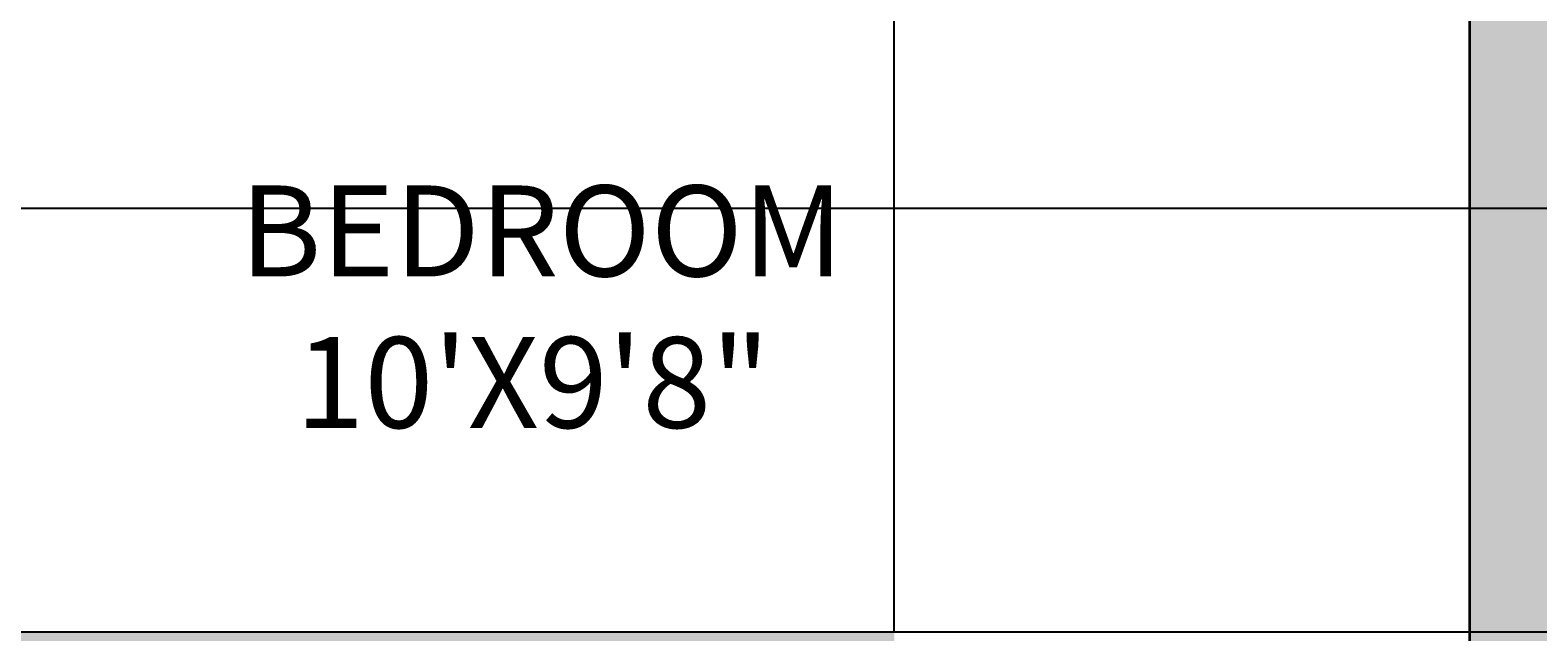
# Model space of a CAD drawing. Units: inches. Extents: x 311 to 815, y -527 to 136.
# Tile 18 of 21: x 444 to 544, y -103 to -63. Entities that reach past the tile are written whole.
import ezdxf

# ---------------------------------------------------------------- set-up
doc = ezdxf.new("R2010")
doc.units = ezdxf.units.IN
doc.header["$MEASUREMENT"] = 0
for name, color, linetype, lineweight in [('A-ANNO-DIMS', 1, 'Continuous', 18), ('A-AREA-IDEN', 8, 'Continuous', 18), ('A-WALL-PATT', 242, 'Continuous', 13), ('wall', 1, 'Continuous', 35)]:
    doc.layers.add(name, color=color, linetype=linetype, lineweight=lineweight)
doc.styles.get("Standard").update_dxf_attribs({"font": 'arial.ttf'})
doc.dimstyles.get("Standard").update_dxf_attribs({"dimtxt": 0.18, "dimasz": 0.18, "dimexe": 0.18, "dimexo": 0.0625, "dimgap": 0.09, "dimtad": 0, "dimtih": 1, "dimtoh": 1, "dimdec": 1, "dimzin": 0, "dimdsep": 46, "dimlunit": 4, "dimtxsty": 'Standard', "dimcen": 0.09, "dimadec": 0, "dimazin": 0, "dimtfac": 1, "dimtdec": 1, "dimtofl": 0, "dimtmove": 0, "dimatfit": 3, "dimfxl": 1, "dimtolj": 1, "dimtzin": 0, "dimarcsym": 0})

# ---------------------------------------------------------------- blocks, each defined once
blk = doc.blocks.new('*D40')
at = {"layer": 'A-ANNO-DIMS', "color": 0, "lineweight": -2, "transparency": 16777216}
for p, q in [((419.385, -75.128), (754.853, -75.128)), ((754.673, -75.308), (754.673, -88.947)), ((754.673, -102.948), (754.673, -89.308)), ((419.385, -103.128), (754.853, -103.128))]:
    blk.add_line(p, q, dxfattribs=at)
at = {"layer": 'A-ANNO-DIMS', "color": 0, "transparency": 16777216}
for points in [[(754.643, -75.308), (754.703, -75.308), (754.673, -75.128)], [(754.643, -102.948), (754.703, -102.948), (754.673, -103.128)]]:
    blk.add_solid(points, dxfattribs=at)
at = {"layer": 'Defpoints', "color": 0, "transparency": 16777216}
for p in [(419.323, -75.128), (419.323, -103.128), (754.673, -103.128)]:
    blk.add_point(p, dxfattribs=at)
at = {"layer": 'A-ANNO-DIMS', "color": 0, "transparency": 16777216, "insert": (754.673, -89.128), "char_height": 0.18, "attachment_point": 5}
blk.add_mtext('\\A1;2\'-4"', dxfattribs=at)
blk = doc.blocks.new('*D51')
at = {"layer": 'A-ANNO-DIMS', "color": 0, "lineweight": -2, "transparency": 16777216}
for p, q in [((501.323, -103.065), (501.323, 54.402)), ((501.503, 54.222), (519.994, 54.222)), ((539.143, 54.222), (520.652, 54.222)), ((539.323, -112.065), (539.323, 54.402))]:
    blk.add_line(p, q, dxfattribs=at)
at = {"layer": 'A-ANNO-DIMS', "color": 0, "transparency": 16777216}
for points in [[(501.503, 54.252), (501.503, 54.192), (501.323, 54.222)], [(539.143, 54.252), (539.143, 54.192), (539.323, 54.222)]]:
    blk.add_solid(points, dxfattribs=at)
at = {"layer": 'Defpoints', "color": 0, "transparency": 16777216}
for p in [(501.323, 54.222), (501.323, -103.128), (539.323, -112.128)]:
    blk.add_point(p, dxfattribs=at)
at = {"layer": 'A-ANNO-DIMS', "color": 0, "transparency": 16777216, "insert": (520.323, 54.222), "char_height": 0.18, "attachment_point": 5}
blk.add_mtext('\\A1;3\'-2"', dxfattribs=at)

msp = doc.modelspace()

# ---------------------------------------------------------------- hatches: boundary and pattern name
at = {"layer": 'A-WALL-PATT'}
h = msp.add_hatch(color=256, dxfattribs=at)
h.dxf.hatch_style = 1
h.paths.add_polyline_path([(557.823, 21.872), (509.323, 21.872), (509.323, 12.872), (539.323, 12.872), (539.323, -112.128), (548.323, -112.128), (548.323, -58.628), (557.823, -58.628), (557.823, -49.628), (548.323, -49.628), (548.323, 12.872), (557.823, 12.872)])
h.paths.add_polyline_path([(449.323, 21.872), (410.323, 21.872), (410.323, -15.128), (419.323, -15.128), (419.323, 12.872), (449.323, 12.872)])
h.paths.add_polyline_path([(626.823, 21.872), (581.823, 21.872), (581.823, 12.872), (591.323, 12.872), (591.323, -49.628), (581.823, -49.628), (581.823, -58.628), (591.323, -58.628), (591.323, -112.128), (600.323, -112.128), (600.323, 12.872), (626.823, 12.872)])
h.paths.add_polyline_path([(722.323, 21.872), (686.823, 21.872), (686.823, 12.872), (713.323, 12.872), (713.323, -18.128), (722.323, -18.128)])
h.paths.add_polyline_path([(722.323, -42.128), (713.323, -42.128), (713.323, -73.128), (722.323, -73.128)])
h.paths.add_polyline_path([(501.323, -103.128), (419.323, -103.128), (419.323, -75.128), (410.323, -75.128), (410.323, -126.628), (419.323, -126.628), (419.323, -112.128), (492.323, -112.128), (492.323, -143.128), (501.323, -143.128)])
h.paths.add_polyline_path([(548.323, -165.128), (419.323, -165.128), (419.323, -150.628), (410.323, -150.628), (410.323, -202.128), (419.323, -202.128), (419.323, -174.128), (548.323, -174.128)])
h.paths.add_polyline_path([(722.323, -103.128), (636.323, -103.128), (636.323, -112.128), (713.323, -112.128), (713.323, -140.128), (722.323, -140.128)])
h.paths.add_polyline_path([(548.323, -210.128), (539.323, -210.128), (539.323, -290.128), (419.323, -290.128), (419.323, -262.128), (410.323, -262.128), (410.323, -311.568), (419.323, -311.568), (419.323, -299.128), (469.323, -299.128), (469.323, -348.128), (443.323, -348.128), (443.323, -357.128), (478.323, -357.128), (478.323, -299.128), (548.323, -299.128)])
h.paths.add_polyline_path([(722.323, -200.128), (713.323, -200.128), (713.323, -228.128), (609.323, -228.128), (609.323, -237.128), (713.323, -237.128), (713.323, -262.628), (722.323, -262.628)])
h.paths.add_polyline_path([(722.323, -322.628), (713.323, -322.628), (713.323, -348.128), (633.323, -348.128), (633.323, -357.128), (713.323, -357.128), (713.323, -385.128), (722.323, -385.128)])
h.paths.add_polyline_path([(419.323, -335.568), (410.323, -335.568), (410.323, -390.84), (419.323, -390.84)])
h.paths.add_polyline_path([(419.323, -450.84), (410.323, -450.84), (410.323, -482.128), (449.323, -482.128), (449.323, -473.128), (419.323, -473.128)])
h.paths.add_polyline_path([(582.823, -473.128), (548.323, -473.128), (548.323, -348.128), (539.323, -348.128), (539.323, -473.128), (509.323, -473.128), (509.323, -482.128), (582.823, -482.128)])
h.paths.add_polyline_path([(722.323, -445.128), (713.323, -445.128), (713.323, -473.128), (678.823, -473.128), (678.823, -482.128), (722.323, -482.128)])

# ---------------------------------------------------------------- linework, layer by layer
at = {"layer": 'wall'}
msp.add_line((539.323, -112.128), (539.323, 12.872), dxfattribs=at)
msp.add_line((539.323, -112.128), (539.323, 12.872), dxfattribs=at)

# ---------------------------------------------------------------- texts
at = {"layer": 'A-AREA-IDEN', "insert": (450.766, -73.637), "char_height": 6.00733, "attachment_point": 1}
msp.add_mtext_dynamic_manual_height_columns('    BEDROOM\\P      10\'X9\'8"', width=59.05986, gutter_width=1.001, heights=[0], dxfattribs=at)

# ---------------------------------------------------------------- dimensions: what is measured, and where the dimension line sits
at = {"layer": 'A-ANNO-DIMS'}
dim = msp.add_linear_dim(base=(501.323, 54.222), p1=(539.323, -112.128), p2=(501.323, -103.128), dimstyle='Standard', override={"dimdec": 1, "dimlfac": 1, "dimrnd": 0, "dimzin": 1, "dimdsep": 46, "dimlunit": 4, "dimfrac": 2}, dxfattribs=at)
dim.commit()
dim.dimension.update_dxf_attribs({"geometry": '*D51', "text_midpoint": (520.323, 54.222)})
dim = msp.add_linear_dim(base=(754.673, -103.128), p1=(419.323, -75.128), p2=(419.323, -103.128), angle=90, dimstyle='Standard', override={"dimdec": 1, "dimlfac": 1, "dimrnd": 0, "dimzin": 1, "dimdsep": 46, "dimlunit": 4, "dimfrac": 2}, dxfattribs=at)
dim.commit()
dim.dimension.update_dxf_attribs({"geometry": '*D40', "text_midpoint": (754.673, -89.128)})

doc.saveas('drawing.dxf')
